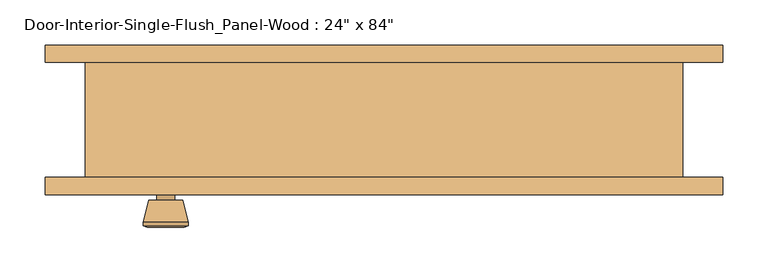
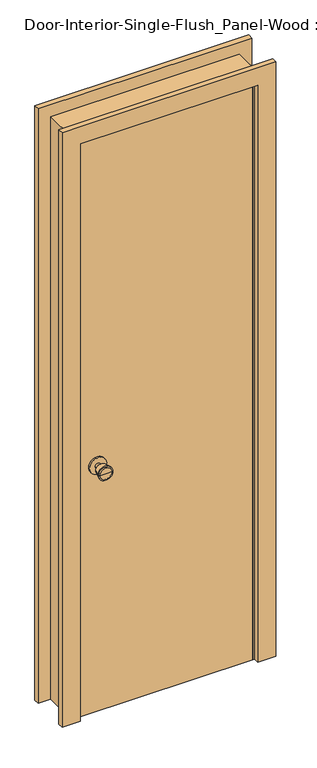
"""IFC4 building model written with IfcOpenShell, lengths in millimetres: door geometry."""

from ifc_helpers import new_model, si_unit, point, frame, frame_2d, origin, origin_with_axes, place, context, project, spatial, polyline, circle_curve, trimmed, segment, composite_curve, outline, extrude, faceted_brep, source, transform, mapped, element, save
from ifc_brep_helpers import plane_surface, cylinder_surface, revolved_surface, advanced_brep


def door_428b1ac9(model_context):
    return source(origin(), model_context, "Body", "SolidModel", [
        advanced_brep(
        [(-241.3, -19.4, 914.4), (-251.3, -19.4, 914.4), (-231.3, -19.4, 914.4), (-220.8241324, 29.6, 914.4), (-261.7758676, 29.6, 914.4), (-241.3, 29.6, 914.4), (-216.3, 27.7721319, 914.4), (-266.3, 27.7721319, 914.4), (-216.3, 24.3084537, 914.4), (-266.3, 24.3084537, 914.4), (-222.663764, -0.4, 914.4), (-259.936236, -0.4, 914.4), (-231.3, -0.4, 914.4), (-251.3, -0.4, 914.4)],
        [
            (0, 1),
            (1, 2, circle_curve(frame((-241.3, -19.4, 914.4), z_axis=(0.0, -1.0, 0.0), x_axis=(-1.0, 0.0, 0.0)), 10.0)),
            (2, 0),
            (2, 1, circle_curve(frame((-241.3, -19.4, 914.4), z_axis=(0.0, -1.0, 0.0), x_axis=(-1.0, 0.0, 0.0)), 10.0)),
            (3, 4, circle_curve(frame((-241.3, 29.6, 914.4), z_axis=(0.0, 1.0, 0.0), x_axis=(-1.0, 0.0, 0.0)), 20.4758676)),
            (4, 5),
            (5, 3),
            (4, 3, circle_curve(frame((-241.3, 29.6, 914.4), z_axis=(0.0, 1.0, 0.0), x_axis=(-1.0, 0.0, 0.0)), 20.4758676)),
            (6, 7, circle_curve(frame((-241.3, 27.7721319, 914.4), z_axis=(0.0, 1.0, 0.0), x_axis=(-1.0, 0.0, 0.0)), 25.0)),
            (7, 4),
            (3, 6),
            (7, 6, circle_curve(frame((-241.3, 27.7721319, 914.4), z_axis=(0.0, 1.0, 0.0), x_axis=(-1.0, 0.0, 0.0)), 25.0)),
            (8, 9, circle_curve(frame((-241.3, 24.3084537, 914.4), z_axis=(0.0, 1.0, 0.0), x_axis=(-1.0, 0.0, 0.0)), 25.0)),
            (9, 7),
            (6, 8),
            (9, 8, circle_curve(frame((-241.3, 24.3084537, 914.4), z_axis=(0.0, 1.0, 0.0), x_axis=(-1.0, 0.0, 0.0)), 25.0)),
            (10, 11, circle_curve(frame((-241.3, -0.4, 914.4), z_axis=(0.0, 1.0, 0.0), x_axis=(-1.0, 0.0, 0.0)), 18.636236)),
            (11, 9),
            (8, 10),
            (11, 10, circle_curve(frame((-241.3, -0.4, 914.4), z_axis=(0.0, 1.0, 0.0), x_axis=(-1.0, 0.0, 0.0)), 18.636236)),
            (12, 13, circle_curve(frame((-241.3, -0.4, 914.4), z_axis=(0.0, 1.0, 0.0), x_axis=(-1.0, 0.0, 0.0)), 10.0)),
            (13, 11),
            (10, 12),
            (13, 12, circle_curve(frame((-241.3, -0.4, 914.4), z_axis=(0.0, 1.0, 0.0), x_axis=(-1.0, 0.0, 0.0)), 10.0)),
            (1, 13),
            (12, 2),
        ],
        [
            plane_surface(frame((-241.3, -19.4, 914.4), z_axis=(0.0, -1.0, 0.0), x_axis=(-1.0, 0.0, 0.0))),
            plane_surface(frame((-241.3, 29.6, 914.4), z_axis=(0.0, 1.0, 0.0), x_axis=(-1.0, 0.0, 0.0))),
            revolved_surface(polyline([(-261.7758676, 29.6, 914.4), (-266.3, 27.7721319, 914.4)]), (-241.3, -19.4, 914.4), (0.0, -1.0, 0.0)),
            cylinder_surface(frame((-241.3, -19.4, 914.4), z_axis=(0.0, -1.0, 0.0), x_axis=(-1.0, 0.0, 0.0)), 25.0),
            revolved_surface(polyline([(-266.3, 24.3084537, 914.4), (-259.936236, -0.4, 914.4)]), (-241.3, -19.4, 914.4), (0.0, -1.0, 0.0)),
            plane_surface(frame((-241.3, -0.4, 914.4), z_axis=(0.0, -1.0, 0.0), x_axis=(-1.0, 0.0, 0.0))),
            cylinder_surface(frame((-241.3, -19.4, 914.4), z_axis=(0.0, -1.0, 0.0), x_axis=(-1.0, 0.0, 0.0)), 10.0),
        ],
        [
            (0, [[1, 2, 3]]),
            (0, [[-3, 4, -1]]),
            (1, [[5, 6, 7]]),
            (1, [[8, -7, -6]]),
            (2, [[9, 10, -5, 11]]),
            (2, [[12, -11, -8, -10]]),
            (3, [[13, 14, -9, 15]]),
            (3, [[16, -15, -12, -14]]),
            (4, [[17, 18, -13, 19]]),
            (4, [[20, -19, -16, -18]]),
            (5, [[21, 22, -17, 23]]),
            (5, [[24, -23, -20, -22]]),
            (6, [[-2, 25, -21, 26]]),
            (6, [[-4, -26, -24, -25]]),
        ],
    ),
        extrude(outline(composite_curve([segment(trimmed(circle_curve(frame_2d((914.4, -241.3)), 30.0), [point((914.4, -271.3))], [point((914.4, -211.3))], False, "CARTESIAN"), True, "CONTINUOUS"), segment(trimmed(circle_curve(frame_2d((914.4, -241.3)), 30.0), [point((914.4, -211.3))], [point((914.4, -271.3))], False, "CARTESIAN"), True, "CONTINUOUS")], self_intersect=False)), frame((0.0, -25.4, 0.0), z_axis=(0.0, 1.0, 0.0), x_axis=(0.0, 0.0, 1.0)), (0.0, 0.0, 1.0), 6.0),
        advanced_brep(
        [(-241.3, -66.325, 914.4), (-231.3, -66.325, 914.4), (-251.3, -66.325, 914.4), (-220.8241324, -115.325, 914.4), (-241.3, -115.325, 914.4), (-261.7758676, -115.325, 914.4), (-216.3, -113.4971319, 914.4), (-266.3, -113.4971319, 914.4), (-216.3, -110.0334537, 914.4), (-266.3, -110.0334537, 914.4), (-222.663764, -85.325, 914.4), (-259.936236, -85.325, 914.4), (-231.3, -85.325, 914.4), (-251.3, -85.325, 914.4)],
        [
            (0, 1),
            (1, 2, circle_curve(frame((-241.3, -66.325, 914.4), z_axis=(0.0, 1.0, 0.0), x_axis=(-1.0, 0.0, 0.0)), 10.0)),
            (2, 0),
            (2, 1, circle_curve(frame((-241.3, -66.325, 914.4), z_axis=(0.0, 1.0, 0.0), x_axis=(-1.0, 0.0, 0.0)), 10.0)),
            (3, 4),
            (4, 5),
            (5, 3, circle_curve(frame((-241.3, -115.325, 914.4), z_axis=(0.0, -1.0, 0.0), x_axis=(-1.0, 0.0, 0.0)), 20.4758676)),
            (3, 5, circle_curve(frame((-241.3, -115.325, 914.4), z_axis=(0.0, -1.0, 0.0), x_axis=(-1.0, 0.0, 0.0)), 20.4758676)),
            (6, 3),
            (5, 7),
            (7, 6, circle_curve(frame((-241.3, -113.4971319, 914.4), z_axis=(0.0, -1.0, 0.0), x_axis=(-1.0, 0.0, 0.0)), 25.0)),
            (6, 7, circle_curve(frame((-241.3, -113.4971319, 914.4), z_axis=(0.0, -1.0, 0.0), x_axis=(-1.0, 0.0, 0.0)), 25.0)),
            (8, 6),
            (7, 9),
            (9, 8, circle_curve(frame((-241.3, -110.0334537, 914.4), z_axis=(0.0, -1.0, 0.0), x_axis=(-1.0, 0.0, 0.0)), 25.0)),
            (8, 9, circle_curve(frame((-241.3, -110.0334537, 914.4), z_axis=(0.0, -1.0, 0.0), x_axis=(-1.0, 0.0, 0.0)), 25.0)),
            (10, 8),
            (9, 11),
            (11, 10, circle_curve(frame((-241.3, -85.325, 914.4), z_axis=(0.0, -1.0, 0.0), x_axis=(-1.0, 0.0, 0.0)), 18.636236)),
            (10, 11, circle_curve(frame((-241.3, -85.325, 914.4), z_axis=(0.0, -1.0, 0.0), x_axis=(-1.0, 0.0, 0.0)), 18.636236)),
            (12, 10),
            (11, 13),
            (13, 12, circle_curve(frame((-241.3, -85.325, 914.4), z_axis=(0.0, -1.0, 0.0), x_axis=(-1.0, 0.0, 0.0)), 10.0)),
            (12, 13, circle_curve(frame((-241.3, -85.325, 914.4), z_axis=(0.0, -1.0, 0.0), x_axis=(-1.0, 0.0, 0.0)), 10.0)),
            (1, 12),
            (13, 2),
        ],
        [
            plane_surface(frame((-241.3, -66.325, 914.4), z_axis=(0.0, 1.0, 0.0), x_axis=(-1.0, 0.0, 0.0))),
            plane_surface(frame((-241.3, -115.325, 914.4), z_axis=(0.0, -1.0, 0.0), x_axis=(-1.0, 0.0, 0.0))),
            revolved_surface(polyline([(-261.7758676, -115.325, 914.4), (-266.3, -113.4971319, 914.4)]), (-241.3, -66.325, 914.4), (0.0, 1.0, 0.0)),
            cylinder_surface(frame((-241.3, -66.325, 914.4), z_axis=(0.0, 1.0, 0.0), x_axis=(-1.0, 0.0, 0.0)), 25.0),
            revolved_surface(polyline([(-266.3, -110.0334537, 914.4), (-259.936236, -85.325, 914.4)]), (-241.3, -66.325, 914.4), (0.0, 1.0, 0.0)),
            plane_surface(frame((-241.3, -85.325, 914.4), z_axis=(0.0, 1.0, 0.0), x_axis=(-1.0, 0.0, 0.0))),
            cylinder_surface(frame((-241.3, -66.325, 914.4), z_axis=(0.0, 1.0, 0.0), x_axis=(-1.0, 0.0, 0.0)), 10.0),
        ],
        [
            (0, [[1, 2, 3]]),
            (0, [[-3, 4, -1]]),
            (1, [[5, 6, 7]]),
            (1, [[-6, -5, 8]]),
            (2, [[9, -7, 10, 11]]),
            (2, [[-10, -8, -9, 12]]),
            (3, [[13, -11, 14, 15]]),
            (3, [[-14, -12, -13, 16]]),
            (4, [[17, -15, 18, 19]]),
            (4, [[-18, -16, -17, 20]]),
            (5, [[21, -19, 22, 23]]),
            (5, [[-22, -20, -21, 24]]),
            (6, [[25, -23, 26, -2]]),
            (6, [[-26, -24, -25, -4]]),
        ],
    ),
        extrude(outline(composite_curve([segment(trimmed(circle_curve(frame_2d((914.4, -241.3)), 30.0), [point((914.4, -271.3))], [point((914.4, -211.3))], False, "CARTESIAN"), True, "CONTINUOUS"), segment(trimmed(circle_curve(frame_2d((914.4, -241.3)), 30.0), [point((914.4, -211.3))], [point((914.4, -271.3))], False, "CARTESIAN"), True, "CONTINUOUS")], self_intersect=False)), frame((0.0, -66.325, 0.0), z_axis=(0.0, 1.0, 0.0), x_axis=(0.0, 0.0, 1.0)), (0.0, 0.0, 1.0), 6.0),
        faceted_brep([(330.2, -60.325, 0.0), (304.8, -60.325, 0.0), (304.8, -25.4, 0.0), (292.1, -25.4, 0.0), (292.1, 9.525, 0.0), (304.8, 9.525, 0.0), (304.8, 66.675, 0.0), (330.2, 66.675, 0.0), (330.2, 66.675, 2159.0), (330.2, -60.325, 2159.0), (304.8, 66.675, 2133.6), (-304.8, 66.675, 2133.6), (-304.8, 66.675, 0.0), (-330.2, 66.675, 0.0), (-330.2, 66.675, 2159.0), (304.8, 9.525, 2133.6), (292.1, 9.525, 2120.9), (-292.1, 9.525, 2120.9), (-292.1, 9.525, 0.0), (-304.8, 9.525, 0.0), (-304.8, 9.525, 2133.6), (292.1, -25.4, 2120.9), (304.8, -25.4, 2133.6), (-304.8, -25.4, 2133.6), (-304.8, -25.4, 0.0), (-292.1, -25.4, 0.0), (-292.1, -25.4, 2120.9), (304.8, -60.325, 2133.6), (-330.2, -60.325, 2159.0), (-330.2, -60.325, 0.0), (-304.8, -60.325, 0.0), (-304.8, -60.325, 2133.6)], [[[0, 1, 2, 3, 4, 5, 6, 7]], [[7, 8, 9, 0]], [[6, 10, 11, 12, 13, 14, 8, 7]], [[5, 15, 10, 6]], [[4, 16, 17, 18, 19, 20, 15, 5]], [[3, 21, 16, 4]], [[2, 22, 23, 24, 25, 26, 21, 3]], [[1, 27, 22, 2]], [[0, 9, 28, 29, 30, 31, 27, 1]], [[8, 14, 28, 9]], [[15, 20, 11, 10]], [[21, 26, 17, 16]], [[27, 31, 23, 22]], [[29, 13, 12, 19, 18, 25, 24, 30]], [[14, 13, 29, 28]], [[20, 19, 12, 11]], [[26, 25, 18, 17]], [[31, 30, 24, 23]]]),
        extrude(outline(polyline([(304.8, -25.4), (304.8, -60.325), (-304.8, -60.325), (-304.8, -25.4), (304.8, -25.4)])), origin_with_axes(), (0.0, 0.0, 1.0), 2133.6),
        extrude(outline(polyline([(0.0, 374.65), (2203.45, 374.65), (2203.45, -374.65), (0.0, -374.65), (0.0, -311.15), (2139.95, -311.15), (2139.95, 311.15), (0.0, 311.15), (0.0, 374.65)])), frame((0.0, -79.375, 0.0), z_axis=(0.0, 1.0, 0.0), x_axis=(0.0, 0.0, 1.0)), (0.0, 0.0, 1.0), 19.05),
        extrude(outline(polyline([(0.0, 374.65), (2203.45, 374.65), (2203.45, -374.65), (0.0, -374.65), (0.0, -311.15), (2139.95, -311.15), (2139.95, 311.15), (0.0, 311.15), (0.0, 374.65)])), frame((0.0, 66.675, 0.0), z_axis=(0.0, 1.0, 0.0), x_axis=(0.0, 0.0, 1.0)), (0.0, 0.0, 1.0), 19.05),
    ])


if __name__ == "__main__":
    model = new_model("IFC4")
    model_context = context("Model", 3, world=origin())
    ifc_project = project(units=[si_unit("LENGTHUNIT", "METRE", prefix="MILLI")], contexts=[model_context])
    site = spatial("IfcSite", under=ifc_project)
    building = spatial("IfcBuilding", under=site)
    placement = place(None, origin())
    door_shape = door_428b1ac9(model_context)
    element("IfcDoor", 1, ObjectType="Door-Interior-Single-Flush_Panel-Wood : 24\" x 84\"", at=placement, inside=building, context=model_context, shape_type="MappedRepresentation", body=[
        mapped(door_shape, transform((0.0, 0.0, 0.0), x_axis=(1.0, 0.0, 0.0), y_axis=(0.0, 1.0, 0.0), z_axis=(0.0, 0.0, 1.0))),
    ])
    save(model, "model.ifc")

# Revit data of these elements
# Type "Door-Interior-Single-Flush_Panel-Wood : 24\" x 84\""
#   Type Mark = "11"
#   Assembly Code = "C1020300"
#   Analytic Construction = "Wooden"
#   Thickness = 0' - 1 3/8"
#   Thermal Resistance (R) = 2.5876 (h·ft²·°F)/BTU
#   Swing Angle [instance default] = 90.00°
#   Rough Width = 2' - 2"
#   Rough Height = 7' - 1"
#   Height = 7' - 0"
#   Width = 2' - 0"
#   Heat Transfer Coefficient (U) = 0.3865 BTU/(h·ft²·°F)
#   Trim Material = Cherry
#   Panel Material = Cherry
#   Frame Material = Cherry
#   Door Handle Material = Aluminum
#   Visual Light Transmittance = 0
#   Solar Heat Gain Coefficient = 0
#   Wall Closure = (empty or 0)
#   Function = (empty or 0)
# Element 1 (IfcDoor, "Door-Interior-Single-Flush_Panel-Wood : 24\" x 84\"")
#   Materials on its faces: "Cherry", "Aluminum"
# Materials
#   "Cherry": class "Wood", colour RGB 226 177 128, transparency 0, Description = "Prunus Serotina", Cost = 0
#   "Aluminum": class "Metal", colour RGB 247 247 247, transparency 0, Description = "Aluminum 6061", Cost = 0
